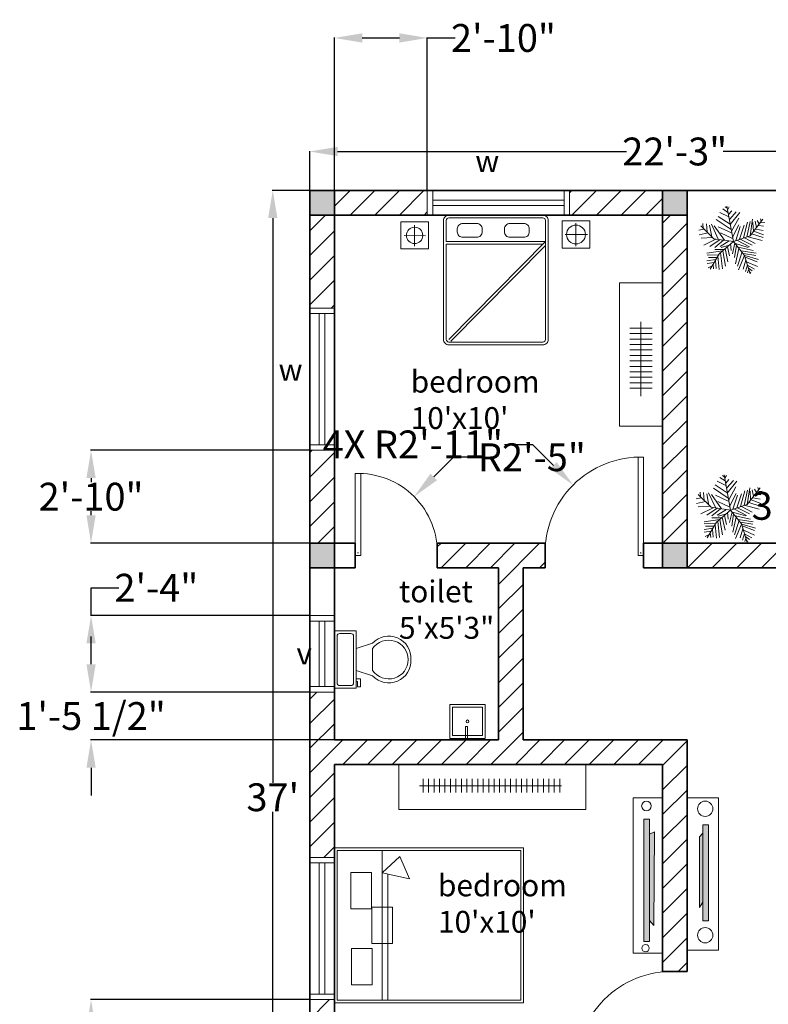
# Model space of a CAD drawing. Units: inches. Extents: x 1222 to 2611, y 176 to 793.
# Tile 2 of 5: x 1223 to 1497, y 433 to 793. Entities that reach past the tile are written whole.
import ezdxf

# ---------------------------------------------------------------- set-up
doc = ezdxf.new("R2010")
doc.units = ezdxf.units.IN
doc.header["$MEASUREMENT"] = 0
for name, color, linetype, lineweight in [('A-ANNO-DIMS', 2, 'Continuous', 18), ('A-ANNO-TEXT', 7, 'Continuous', 25), ('A-AREA-IDEN', 7, 'Continuous', 25), ('A-COLS', 7, 'Continuous', 35), ('A-COLS-PATT', 18, 'Continuous', 13), ('A-DOOR', 3, 'Continuous', 18), ('A-EQPM', 8, 'Continuous', 18), ('A-EQPM-PATT', 18, 'Continuous', 13), ('A-FLOR-CASE', 9, 'Continuous', 18), ('A-FLOR-FIXT', 9, 'Continuous', 18), ('A-FURN', 8, 'Continuous', 18), ('A-GLAZ', 4, 'Continuous', 18), ('A-WALL', 7, 'Continuous', 35), ('A-WALL-PATT', 30, 'Continuous', 13), ('L-PLNT', 94, 'Continuous', 13)]:
    doc.layers.add(name, color=color, linetype=linetype, lineweight=lineweight)
doc.styles.get("Standard").update_dxf_attribs({"font": 'arial.ttf'})
doc.dimstyles.get("Standard").update_dxf_attribs({"dimtxt": 10.18, "dimasz": 10.18, "dimexe": 0.18, "dimexo": 0.0625, "dimgap": 0.09, "dimtad": 0, "dimtih": 1, "dimtoh": 1, "dimdec": 0, "dimzin": 0, "dimdsep": 46, "dimlunit": 3, "dimtxsty": 'Standard', "dimcen": 0.09, "dimadec": 0, "dimazin": 0, "dimtfac": 1, "dimtdec": 0, "dimtofl": 0, "dimtmove": 0, "dimatfit": 3, "dimfxl": 1, "dimtolj": 1, "dimtzin": 0, "dimarcsym": 0})

# ---------------------------------------------------------------- blocks, each defined once
blk = doc.blocks.new('*U2')
for p, q in [((9.5, -6), (9.5, -2)), ((-10, -8.5), (-8, -8.5)), ((-10, -9.5), (-10, -8.5)), ((-7, -9.5), (-10, -9.5)), ((-8, -8.5), (-8, -8)), ((-7, -8), (-7, -9.5)), ((-4, -8), (-6, -14)), ((4, -8), (6, -14)), ((4, -14), (-4, -14))]:
    blk.add_line(p, q)
blk.add_lwpolyline([(10.5, -8), (10.5, 0), (-10.5, 0), (-10.5, -8)], close=True)
for points in [[(-9.5, -2), (-9.5, -6)], [(8.5, -1), (-8.5, -1)], [(-8.5, -7), (8.5, -7)]]:
    blk.add_lwpolyline(points)
for centre, radius, start, end in [((-8.625, -1.875), 0.8839, 81.8699, 188.1301), ((8.625, -1.875), 0.8839, 351.8699, 98.1301), ((-8.625, -6.125), 0.8839, 171.869898, 278.1301), ((8.625, -6.125), 0.8839, 261.8699, 8.1301), ((-0.4772, -19.9188), 8.0953, 133.01722, 273.38), ((0.0374, -19.8731), 7.127, 124.50543, 269.7), ((-0.0373, -19.8731), 7.127, 270.3, 55.4946), ((0.4773, -19.9188), 8.0953, 266.62, 46.9828)]:
    blk.add_arc(centre, radius, start, end)
blk = doc.blocks.new('*U4')
for p, q in [((-8.737, 47.138), (-17.069, 52.711)), ((-10.186, 53.64), (-13.084, 55.962)), ((0, 0), (-10.5, 57)), ((-9.099, 51.782), (-6.563, 55.962)), ((-7.65, 43.423), (-2.578, 49.46)), ((-5.839, 35.992), (4.667, 48.067)), ((-3.665, 19.273), (-27.574, 35.527)), ((-5.114, 28.097), (-24.676, 40.636)), ((-7.288, 39.707), (-21.778, 46.673)), ((-5.114, 27.632), (10.463, 46.673)), ((-2.941, 16.486), (8.652, 37.85)), ((22.055, 7.198), (27.489, 32.277)), ((27, 9), (48, 36)), ((27.127, 9.056), (31.112, 35.992)), ((35.096, 32.741), (37.27, 22.524)), ((38.719, 34.134), (41.979, 28.561)), ((44.153, 36.456), (45.239, 32.741)), ((-47.498, 19.737), (-55.83, 18.344)), ((-31.5, 4.5), (-52.5, 25.5)), ((-48.585, 21.131), (-49.309, 29.026)), ((-43.513, 28.561), (-42.427, 15.558)), ((-38.442, 26.239), (-34.819, 7.663)), ((-35.544, 28.097), (-24.314, 3.947)), ((-14.533, 2.09), (-30.834, 25.31)), ((-24.314, 23.917), (-2.941, 13.7)), ((-1.129, 6.734), (9.014, 26.704)), ((3.942, 1.625), (11.187, 24.381)), ((10.101, 3.483), (17.708, 26.239)), ((16.259, 5.805), (23.142, 31.348)), ((31.836, 30.883), (32.561, 16.486)), ((33.285, 16.486), (48.862, 10.913)), ((36.183, 19.737), (48.137, 17.88)), ((40.53, 25.775), (48.862, 24.846)), ((43.791, 29.954), (51.036, 30.883)), ((-40.615, 13.7), (-55.105, 10.913)), ((-33.37, 6.269), (-52.207, 5.34)), ((-28.299, 3.483), (-47.86, -5.805)), ((-21.416, 3.018), (-38.079, -8.128)), ((0, 0), (-31.5, 4.5)), ((-15.982, 2.09), (-30.11, -9.521)), ((0, 0), (-22.5, -19.5)), ((-6.563, 1.161), (-21.416, -8.128)), ((-20.691, 13.7), (-1.129, 4.876)), ((0, 0), (27, 9)), ((0, 0), (18, -22.5)), ((6.478, 1.625), (26.04, -8.592)), ((11.187, 3.483), (30.749, -5.805)), ((18.07, 5.805), (35.096, -3.483)), ((24.229, 7.663), (46.688, 1.625)), ((29.662, 12.307), (48.137, 6.269)), ((-17.431, -15.094), (-42.789, -18.809)), ((-15.257, -12.772), (-30.11, -12.772)), ((-6.563, -5.805), (-19.967, -9.985)), ((-17.069, -15.094), (-12.721, -40.172)), ((-13.446, -11.378), (-8.737, -32.741)), ((-9.461, -8.592), (-6.201, -23.453)), ((-4.752, -3.483), (-3.665, -14.629)), ((2.493, -3.019), (-1.491, -20.202)), ((1.769, -2.555), (24.229, -9.521)), ((5.029, -6.27), (2.131, -25.775)), ((9.014, -11.378), (3.58, -35.992)), ((7.565, -9.056), (32.198, -14.629)), ((12.274, -15.094), (36.907, -18.809)), ((-28.299, -29.026), (-42.789, -31.348)), ((-24.314, -21.596), (-42.427, -22.06)), ((-26.849, -26.24), (-40.253, -25.775)), ((-22.5, -19.5), (-37.5, -45)), ((-29.023, -30.884), (-27.936, -43.887)), ((-25.038, -23.918), (-22.865, -45.281)), ((-20.691, -18.345), (-17.793, -44.352)), ((14.085, -16.951), (6.478, -40.172)), ((18.07, -22.524), (8.289, -45.745)), ((20.244, -30.419), (15.897, -44.816)), ((16.259, -19.738), (36.183, -22.989)), ((18, -22.5), (27, -52.5)), ((18.433, -22.524), (40.53, -29.026)), ((19.157, -25.311), (38.719, -33.206)), ((-30.834, -34.135), (-42.427, -35.528)), ((-34.457, -39.708), (-40.978, -42.494)), ((-32.646, -36.921), (-31.921, -44.352)), ((22.78, -37.85), (19.519, -48.532)), ((21.331, -32.741), (39.081, -40.636)), ((22.78, -38.314), (34.372, -44.816)), ((24.591, -45.745), (23.142, -50.854)), ((24.591, -43.423), (30.749, -47.603)), ((26.764, -49.925), (28.213, -50.854))]:
    blk.add_line(p, q)
blk = doc.blocks.new('*D9')
at = {"layer": 'A-ANNO-DIMS', "color": 0, "lineweight": -2, "transparency": 16777216}
for p, q in [((1328.8, 730.54), (1328.8, 744.93)), ((1338.98, 744.75), (1444.64, 744.75)), ((1585.62, 744.75), (1479.97, 744.75)), ((1595.8, 730.54), (1595.8, 744.93))]:
    blk.add_line(p, q, dxfattribs=at)
at = {"layer": 'A-ANNO-DIMS', "color": 0, "transparency": 16777216}
for points in [[(1338.98, 746.45), (1338.98, 743.05), (1328.8, 744.75)], [(1585.62, 746.45), (1585.62, 743.05), (1595.8, 744.75)]]:
    blk.add_solid(points, dxfattribs=at)
at = {"layer": 'Defpoints', "color": 0, "transparency": 16777216}
for p in [(1595.8, 744.75), (1328.8, 730.47), (1595.8, 730.47)]:
    blk.add_point(p, dxfattribs=at)
at = {"layer": 'A-ANNO-DIMS', "color": 0, "transparency": 16777216, "insert": (1462.3, 744.75), "char_height": 10.18, "attachment_point": 5}
blk.add_mtext('\\A1;22\'-3"', dxfattribs=at)
blk = doc.blocks.new('*D10')
at = {"layer": 'A-ANNO-DIMS', "color": 0, "lineweight": -2, "transparency": 16777216}
for p, q in [((1328.74, 730.54), (1315.1, 730.54)), ((1315.28, 720.36), (1315.28, 513.8)), ((1315.28, 296.65), (1315.28, 503.21)), ((1328.74, 286.47), (1315.1, 286.47))]:
    blk.add_line(p, q, dxfattribs=at)
at = {"layer": 'A-ANNO-DIMS', "color": 0, "transparency": 16777216}
for points in [[(1313.58, 720.36), (1316.97, 720.36), (1315.28, 730.54)], [(1313.58, 296.65), (1316.97, 296.65), (1315.28, 286.47)]]:
    blk.add_solid(points, dxfattribs=at)
at = {"layer": 'Defpoints', "color": 0, "transparency": 16777216}
for p in [(1315.28, 730.54), (1328.8, 730.54), (1328.8, 286.47)]:
    blk.add_point(p, dxfattribs=at)
at = {"layer": 'A-ANNO-DIMS', "color": 0, "transparency": 16777216, "insert": (1315.28, 508.5), "char_height": 10.18, "attachment_point": 5}
blk.add_mtext("\\A1;37'", dxfattribs=at)
blk = doc.blocks.new('DOOR-SWING-36IN')
for p, q in [((34.01, 0), (34.01, 36)), ((36.01, 0), (36.01, 36)), ((34.01, 0), (36.01, 0))]:
    blk.add_line(p, q)
blk.add_arc((35.01, 1), 35.01, 88.3634, 181.6366)
blk = doc.blocks.new('WINDOW-48IN-PLAN')
for p, q in [((0, 0), (0, 9)), ((2, 0), (2, 9)), ((50, 0), (50, 9)), ((52, 0), (52, 9)), ((2, 5.5), (50, 5.5)), ((2, 3.5), (50, 3.5))]:
    blk.add_line(p, q)
blk = doc.blocks.new('COLUMN-9X9IN')
blk.add_lwpolyline([(0, 9), (9, 9), (9, 0), (0, 0)], close=True)
blk = doc.blocks.new('*D21')
at = {"layer": 'A-ANNO-DIMS', "color": 0, "lineweight": -2, "transparency": 16777216}
for p, q in [((1538.86, 633.25), (1533.3, 633.25)), ((1533.48, 623.07), (1533.48, 620.47)), ((1533.48, 607.15), (1533.48, 609.75)), ((1538.86, 596.97), (1533.3, 596.97))]:
    blk.add_line(p, q, dxfattribs=at)
at = {"layer": 'A-ANNO-DIMS', "color": 0, "transparency": 16777216}
for points in [[(1531.79, 623.07), (1535.18, 623.07), (1533.48, 633.25)], [(1531.79, 607.15), (1535.18, 607.15), (1533.48, 596.97)]]:
    blk.add_solid(points, dxfattribs=at)
at = {"layer": 'Defpoints', "color": 0, "transparency": 16777216}
for p in [(1533.48, 633.25), (1538.92, 633.25), (1538.92, 596.97)]:
    blk.add_point(p, dxfattribs=at)
at = {"layer": 'A-ANNO-DIMS', "color": 0, "transparency": 16777216, "insert": (1533.48, 615.11), "char_height": 10.18, "attachment_point": 5}
blk.add_mtext('\\A1;3\'-0 1/2" TYP.', dxfattribs=at)
blk = doc.blocks.new('*D30')
at = {"layer": 'A-ANNO-DIMS', "color": 0, "lineweight": -2, "transparency": 16777216}
for p, q in [((1337.8, 721.54), (1337.8, 786.47)), ((1347.98, 786.29), (1361.62, 786.29)), ((1371.8, 730.54), (1371.8, 786.47)), ((1371.8, 786.29), (1381.98, 786.29))]:
    blk.add_line(p, q, dxfattribs=at)
at = {"layer": 'A-ANNO-DIMS', "color": 0, "transparency": 16777216}
for points in [[(1347.98, 787.99), (1347.98, 784.59), (1337.8, 786.29)], [(1361.62, 787.99), (1361.62, 784.59), (1371.8, 786.29)]]:
    blk.add_solid(points, dxfattribs=at)
at = {"layer": 'Defpoints', "color": 0, "transparency": 16777216}
for p in [(1371.8, 786.29), (1371.8, 730.47), (1337.8, 721.47)]:
    blk.add_point(p, dxfattribs=at)
at = {"layer": 'A-ANNO-DIMS', "color": 0, "transparency": 16777216, "insert": (1399.65, 786.29), "char_height": 10.18, "attachment_point": 5}
blk.add_mtext('\\A1;2\'-10"', dxfattribs=at)
blk = doc.blocks.new('*D31')
at = {"layer": 'A-ANNO-DIMS', "color": 0, "lineweight": -2, "transparency": 16777216}
for p, q in [((1328.74, 635.47), (1248.62, 635.47)), ((1248.8, 625.29), (1248.8, 623.76)), ((1248.8, 611.65), (1248.8, 613.19)), ((1328.74, 601.47), (1248.62, 601.47))]:
    blk.add_line(p, q, dxfattribs=at)
at = {"layer": 'A-ANNO-DIMS', "color": 0, "transparency": 16777216}
for points in [[(1247.11, 625.29), (1250.5, 625.29), (1248.8, 635.47)], [(1247.11, 611.65), (1250.5, 611.65), (1248.8, 601.47)]]:
    blk.add_solid(points, dxfattribs=at)
at = {"layer": 'Defpoints', "color": 0, "transparency": 16777216}
for p in [(1248.8, 635.47), (1328.8, 635.47), (1328.8, 601.47)]:
    blk.add_point(p, dxfattribs=at)
at = {"layer": 'A-ANNO-DIMS', "color": 0, "transparency": 16777216, "insert": (1248.8, 618.47), "char_height": 10.18, "attachment_point": 5}
blk.add_mtext('\\A1;2\'-10"', dxfattribs=at)
blk = doc.blocks.new('*D32')
at = {"layer": 'A-ANNO-DIMS', "color": 0, "lineweight": -2, "transparency": 16777216}
for p, q in [((1248.8, 557.15), (1248.8, 567.33)), ((1328.74, 546.97), (1248.62, 546.97)), ((1337.74, 529.47), (1248.62, 529.47)), ((1248.8, 519.29), (1248.8, 509.11))]:
    blk.add_line(p, q, dxfattribs=at)
at = {"layer": 'A-ANNO-DIMS', "color": 0, "transparency": 16777216}
for points in [[(1247.11, 557.15), (1250.5, 557.15), (1248.8, 546.97)], [(1247.11, 519.29), (1250.5, 519.29), (1248.8, 529.47)]]:
    blk.add_solid(points, dxfattribs=at)
at = {"layer": 'Defpoints', "color": 0, "transparency": 16777216}
for p in [(1248.8, 546.97), (1328.8, 546.97), (1337.8, 529.47)]:
    blk.add_point(p, dxfattribs=at)
at = {"layer": 'A-ANNO-DIMS', "color": 0, "transparency": 16777216, "insert": (1248.8, 538.22), "char_height": 10.18, "attachment_point": 5}
blk.add_mtext('\\A1;1\'-5 1/2"', dxfattribs=at)
blk = doc.blocks.new('*D33')
at = {"layer": 'A-ANNO-DIMS', "color": 0, "lineweight": -2, "transparency": 16777216}
for p, q in [((1248.8, 574.97), (1248.8, 585.15)), ((1248.8, 585.15), (1258.98, 585.15)), ((1328.74, 574.97), (1248.62, 574.97)), ((1248.8, 557.15), (1248.8, 564.79)), ((1328.74, 546.97), (1248.62, 546.97))]:
    blk.add_line(p, q, dxfattribs=at)
at = {"layer": 'A-ANNO-DIMS', "color": 0, "transparency": 16777216}
for points in [[(1247.11, 564.79), (1250.5, 564.79), (1248.8, 574.97)], [(1247.11, 557.15), (1250.5, 557.15), (1248.8, 546.97)]]:
    blk.add_solid(points, dxfattribs=at)
at = {"layer": 'Defpoints', "color": 0, "transparency": 16777216}
for p in [(1248.8, 574.97), (1328.8, 574.97), (1328.8, 546.97)]:
    blk.add_point(p, dxfattribs=at)
at = {"layer": 'A-ANNO-DIMS', "color": 0, "transparency": 16777216, "insert": (1272.69, 585.15), "char_height": 10.18, "attachment_point": 5}
blk.add_mtext('\\A1;2\'-4"', dxfattribs=at)
blk = doc.blocks.new('*D34')
at = {"layer": 'A-ANNO-DIMS', "color": 0, "lineweight": -2, "transparency": 16777216}
for p, q in [((1328.74, 434.47), (1248.62, 434.47)), ((1248.8, 424.29), (1248.8, 422.76)), ((1248.8, 410.65), (1248.8, 412.19)), ((1328.74, 400.47), (1248.62, 400.47))]:
    blk.add_line(p, q, dxfattribs=at)
at = {"layer": 'A-ANNO-DIMS', "color": 0, "transparency": 16777216}
for points in [[(1247.11, 424.29), (1250.5, 424.29), (1248.8, 434.47)], [(1247.11, 410.65), (1250.5, 410.65), (1248.8, 400.47)]]:
    blk.add_solid(points, dxfattribs=at)
at = {"layer": 'Defpoints', "color": 0, "transparency": 16777216}
for p in [(1248.8, 434.47), (1328.8, 434.47), (1328.8, 400.47)]:
    blk.add_point(p, dxfattribs=at)
at = {"layer": 'A-ANNO-DIMS', "color": 0, "transparency": 16777216, "insert": (1248.8, 417.47), "char_height": 10.18, "attachment_point": 5}
blk.add_mtext('\\A1;2\'-10"', dxfattribs=at)
blk = doc.blocks.new('*D56')
at = {"layer": 'A-ANNO-DIMS', "color": 0, "lineweight": -2, "transparency": 16777216}
for p, q in [((1400.08, 637.59), (1410.26, 637.59)), ((1410.26, 637.59), (1417.91, 629.93)), ((1449.78, 597.97), (1449.96, 597.97)), ((1449.87, 597.88), (1449.87, 598.06))]:
    blk.add_line(p, q, dxfattribs=at)
at = {"layer": 'A-ANNO-DIMS', "color": 0, "transparency": 16777216}
blk.add_solid([(1419.11, 631.13), (1416.71, 628.73), (1425.11, 622.73)], dxfattribs=at)
at = {"layer": 'Defpoints', "color": 0, "transparency": 16777216}
for p in [(1425.11, 622.73), (1449.87, 597.97)]:
    blk.add_point(p, dxfattribs=at)
at = {"layer": 'A-ANNO-DIMS', "color": 0, "transparency": 16777216, "insert": (1366.49, 637.59), "char_height": 10.18, "attachment_point": 5}
blk.add_mtext('\\A1;4X R2\'-11"', dxfattribs=at)
blk = doc.blocks.new('*D57')
at = {"layer": 'A-ANNO-DIMS', "color": 0, "lineweight": -2, "transparency": 16777216}
for p, q in [((1381.37, 632.89), (1374.17, 625.69)), ((1391.55, 632.89), (1381.37, 632.89)), ((1346.36, 597.97), (1346.54, 597.97)), ((1346.45, 597.88), (1346.45, 598.06))]:
    blk.add_line(p, q, dxfattribs=at)
at = {"layer": 'A-ANNO-DIMS', "color": 0, "transparency": 16777216}
blk.add_solid([(1372.97, 626.89), (1375.37, 624.49), (1366.97, 618.49)], dxfattribs=at)
at = {"layer": 'Defpoints', "color": 0, "transparency": 16777216}
for p in [(1366.97, 618.49), (1346.45, 597.97)]:
    blk.add_point(p, dxfattribs=at)
at = {"layer": 'A-ANNO-DIMS', "color": 0, "transparency": 16777216, "insert": (1410.04, 632.89), "char_height": 10.18, "attachment_point": 5}
blk.add_mtext('\\A1;R2\'-5"', dxfattribs=at)

msp = doc.modelspace()

# ---------------------------------------------------------------- hatches: boundary and pattern name
at = {"layer": 'A-COLS-PATT'}
h = msp.add_hatch(color=256, dxfattribs=at)
h.dxf.hatch_style = 1
h.paths.add_polyline_path([(1337.8, 730.47), (1328.8, 730.47), (1328.8, 721.47), (1337.8, 721.47)])
h.paths.add_polyline_path([(1466.8, 730.47), (1457.8, 730.47), (1457.8, 721.47), (1466.8, 721.47)])
h.paths.add_polyline_path([(1595.8, 730.47), (1586.8, 730.47), (1586.8, 721.47), (1595.8, 721.47)])
h.paths.add_polyline_path([(1595.8, 601.42), (1586.8, 601.42), (1586.8, 592.42), (1595.8, 592.42)])
h.paths.add_polyline_path([(1466.8, 601.47), (1457.8, 601.47), (1457.8, 592.47), (1466.8, 592.47)])
h.paths.add_polyline_path([(1337.8, 601.47), (1328.8, 601.47), (1328.8, 592.47), (1337.8, 592.47)])
h.paths.add_polyline_path([(1337.8, 400.47), (1328.8, 400.47), (1328.8, 391.47), (1337.8, 391.47)])
h.paths.add_polyline_path([(1466.8, 400.47), (1457.8, 400.47), (1457.8, 391.47), (1466.8, 391.47)])
h.paths.add_polyline_path([(1595.8, 400.41), (1586.8, 400.41), (1586.8, 391.41), (1595.8, 391.41)])
h.paths.add_polyline_path([(1466.56, 295.47), (1457.56, 295.47), (1457.56, 286.47), (1466.56, 286.47)])
h.paths.add_polyline_path([(1595.8, 295.47), (1586.8, 295.47), (1586.8, 286.47), (1595.8, 286.47)])
h.paths.add_polyline_path([(1337.8, 295.47), (1328.8, 295.47), (1328.8, 286.47), (1337.8, 286.47)])
at = {"layer": 'A-EQPM-PATT'}
h = msp.add_hatch(color=256, dxfattribs=at)
h.dxf.hatch_style = 1
h.paths.add_polyline_path([(1453.1, 500.52), (1450.95, 500.52), (1450.95, 455.73), (1453.1, 455.73)])
h.paths.add_polyline_path([(1454.95, 495.86), (1453.1, 494.94), (1453.1, 463.37), (1454.68, 461.57)])
h = msp.add_hatch(color=256, dxfattribs=at)
h.dxf.hatch_style = 1
h.paths.add_polyline_path([(1474.66, 498.47), (1472.58, 498.47), (1472.58, 463.24), (1474.66, 463.24)])
h.paths.add_polyline_path([(1472.58, 495.4), (1471.4, 494.01), (1471.4, 468.17), (1472.58, 470.11)])
at = {"layer": 'A-WALL-PATT'}
h = msp.add_hatch(dxfattribs=at)
h.set_pattern_fill('ANSI31', color=256, scale=51)
h.paths.add_polyline_path([(1337.8, 721.47), (1328.8, 721.47), (1328.8, 687.47), (1337.8, 687.47)])
h.paths.add_polyline_path([(1337.8, 635.47), (1328.8, 635.47), (1328.8, 601.47), (1337.8, 601.47)])
h.paths.add_polyline_path([(1371.8, 730.47), (1337.8, 730.47), (1337.8, 721.47), (1371.8, 721.47)])
h.paths.add_polyline_path([(1457.8, 730.47), (1423.8, 730.47), (1423.8, 721.47), (1457.8, 721.47)])
h.paths.add_polyline_path([(1466.8, 721.47), (1457.8, 721.47), (1457.8, 601.47), (1466.8, 601.47)])
h.paths.add_polyline_path([(1539.2, 596.97, -0.014283), (1539.2, 598.97), (1539.2, 601.47), (1466.8, 601.47), (1466.8, 592.47), (1539.2, 592.47)])
h.paths.add_polyline_path([(1595.8, 592.42), (1586.8, 592.42), (1586.8, 534.47), (1595.8, 534.47)])
h.paths.add_polyline_path([(1595.8, 458.47), (1586.8, 458.47), (1586.8, 400.41), (1595.8, 400.41)])
h.paths.add_polyline_path([(1595.8, 391.41), (1586.8, 391.41), (1586.8, 369.47), (1595.8, 369.47)])
h.paths.add_polyline_path([(1595.8, 317.47), (1586.8, 317.47), (1586.8, 295.47), (1595.8, 295.47)])
h.paths.add_polyline_path([(1586.8, 295.47), (1552.8, 295.47), (1552.8, 286.47), (1586.8, 286.47)])
h.paths.add_polyline_path([(1500.8, 295.47), (1466.8, 295.47), (1466.8, 349.72), (1462.3, 349.72, -0.014283), (1460.3, 349.72), (1457.8, 349.72), (1457.8, 295.47), (1466.56, 295.47), (1466.56, 286.47), (1500.8, 286.47)])
h.paths.add_polyline_path([(1457.56, 295.47), (1337.8, 295.47), (1337.8, 286.47), (1457.56, 286.47)])
h.paths.add_polyline_path([(1337.8, 317.47), (1328.8, 317.47), (1328.8, 295.47), (1337.8, 295.47)])
h.paths.add_polyline_path([(1337.8, 391.47), (1328.8, 391.47), (1328.8, 369.47), (1337.8, 369.47)])
h.paths.add_polyline_path([(1337.8, 434.47), (1328.8, 434.47), (1328.8, 400.47), (1337.8, 400.47)])
h.paths.add_polyline_path([(1457.8, 400.47), (1337.8, 400.47), (1337.8, 391.47), (1457.8, 391.47)])
h.paths.add_polyline_path([(1546.8, 395.97, -0.014283), (1546.8, 397.97), (1546.8, 400.47), (1466.8, 400.47), (1466.8, 391.47), (1546.8, 391.47)])
h.paths.add_polyline_path([(1466.8, 408.77), (1457.8, 408.77), (1457.8, 400.47), (1466.8, 400.47)])
h.paths.add_polyline_path([(1466.8, 391.47), (1457.8, 391.47), (1457.8, 385.72), (1466.8, 385.72)])
h.paths.add_polyline_path([(1586.8, 400.47), (1582.8, 400.47), (1582.8, 395.97), (1582.8, 391.47), (1586.8, 391.47)])
h.paths.add_polyline_path([(1466.8, 529.47), (1457.8, 529.47), (1406.8, 529.47), (1406.8, 592.47), (1414.87, 592.47), (1414.87, 596.97, -0.014283), (1414.87, 598.97), (1414.87, 601.47), (1375.45, 601.47), (1375.45, 598.97, -0.017236), (1375.45, 596.97), (1375.45, 592.47), (1397.8, 592.47), (1397.8, 529.47), (1337.8, 529.47), (1337.8, 546.97), (1328.8, 546.97), (1328.8, 486.47), (1337.8, 486.47), (1337.8, 490.02), (1337.8, 520.47), (1457.8, 520.47), (1457.8, 444.77), (1460.3, 444.77, -0.014283), (1462.3, 444.77), (1466.8, 444.77)])
h.paths.add_polyline_path([(1457.8, 601.47), (1450.87, 601.47), (1450.87, 596.97), (1450.87, 592.47), (1457.8, 592.47)], flags=0)
h.paths.add_polyline_path([(1586.8, 601.47), (1575.2, 601.47), (1575.2, 596.97), (1575.2, 592.47), (1586.8, 592.47)])

# ---------------------------------------------------------------- linework, layer by layer
at = {"layer": 'A-DOOR'}
for p, q in [((1345.45, 596.97), (1345.45, 626.97)), ((1347.45, 596.97), (1347.45, 626.97)), ((1347.45, 596.97), (1345.45, 596.97))]:
    msp.add_line(p, q, dxfattribs=at)
msp.add_arc((1346.45, 597.97), 29.02, 358.0251, 91.9749, dxfattribs=at)
at = {"layer": 'A-EQPM'}
for p, q in [((1453.1, 494.94), (1454.95, 495.86)), ((1454.95, 495.86), (1454.68, 461.57)), ((1472.58, 495.4), (1471.4, 494.01)), ((1471.4, 494.01), (1471.4, 468.17)), ((1471.4, 468.17), (1472.58, 470.11)), ((1454.68, 461.57), (1453.1, 463.37))]:
    msp.add_line(p, q, dxfattribs=at)
for points in [[(1457.8, 508.28), (1457.8, 508.28), (1447.11, 508.28), (1447.11, 508.28), (1447.11, 451.46), (1447.11, 451.46), (1457.8, 451.46), (1457.8, 451.46)], [(1466.8, 508.28), (1466.8, 508.28), (1478.29, 508.28), (1478.29, 508.28), (1478.29, 452.6), (1478.29, 452.6), (1466.8, 452.6), (1466.8, 452.6)], [(1453.1, 500.52), (1453.1, 500.52), (1450.95, 500.52), (1450.95, 500.52), (1450.95, 455.73), (1450.95, 455.73), (1453.1, 455.73), (1453.1, 455.73)], [(1474.66, 498.47), (1474.66, 498.47), (1472.58, 498.47), (1472.58, 498.47), (1472.58, 463.24), (1472.58, 463.24), (1474.66, 463.24), (1474.66, 463.24)]]:
    msp.add_lwpolyline(points, close=True, dxfattribs=at)
for centre, radius in [((1451.95, 505.32), 1.75), ((1473.43, 504.3), 2.8), ((1473.43, 458.02), 2.8), ((1451.63, 453.31), 1.34)]:
    msp.add_circle(centre, radius, dxfattribs=at)
at = {"layer": 'A-FLOR-CASE'}
for p, q in [((1449.91, 682.43), (1449.91, 655.25)), ((1445.91, 680.13), (1454.06, 680.13)), ((1445.91, 678.13), (1454.06, 678.13)), ((1445.91, 676.13), (1454.06, 676.13)), ((1445.91, 674.13), (1454.06, 674.13)), ((1445.91, 672.13), (1454.06, 672.13)), ((1445.91, 670.13), (1454.06, 670.13)), ((1445.91, 668.13), (1454.06, 668.13)), ((1445.91, 666.13), (1454.06, 666.13)), ((1445.91, 664.13), (1454.06, 664.13)), ((1445.91, 662.13), (1454.06, 662.13)), ((1445.91, 660.13), (1454.06, 660.13)), ((1445.91, 658.13), (1454.06, 658.13)), ((1370.25, 515.22), (1370.25, 510.23)), ((1372.25, 515.22), (1372.25, 510.23)), ((1374.25, 515.22), (1374.25, 510.23)), ((1376.25, 515.22), (1376.25, 510.23)), ((1378.25, 515.22), (1378.25, 510.23)), ((1380.25, 515.22), (1380.25, 510.23)), ((1382.25, 515.22), (1382.25, 510.23)), ((1384.25, 515.22), (1384.25, 510.23)), ((1386.25, 515.22), (1386.25, 510.23)), ((1388.25, 515.22), (1388.25, 510.23)), ((1390.25, 515.22), (1390.25, 510.23)), ((1392.25, 515.22), (1392.25, 510.23)), ((1394.25, 515.22), (1394.25, 510.23)), ((1396.25, 515.22), (1396.25, 510.23)), ((1398.25, 515.22), (1398.25, 510.23)), ((1400.25, 515.22), (1400.25, 510.23)), ((1402.25, 515.22), (1402.25, 510.23)), ((1404.25, 515.22), (1404.25, 510.23)), ((1406.25, 515.22), (1406.25, 510.23)), ((1408.25, 515.22), (1408.25, 510.23)), ((1410.25, 515.22), (1410.25, 510.23)), ((1412.25, 515.22), (1412.25, 510.23)), ((1414.25, 515.22), (1414.25, 510.23)), ((1416.25, 515.22), (1416.25, 510.23)), ((1418.25, 515.22), (1418.25, 510.23)), ((1420.25, 515.22), (1420.25, 510.23)), ((1368.88, 512.68), (1420.85, 512.68))]:
    msp.add_line(p, q, dxfattribs=at)
for points in [[(1457.8, 696.67), (1457.8, 696.67), (1442.08, 696.67), (1442.08, 696.67), (1442.08, 644.23), (1442.08, 644.23), (1457.8, 644.23), (1457.8, 644.23)], [(1442.08, 666.74), (1442.08, 666.74), (1442.08, 666.74), (1442.08, 666.74), (1442.08, 660.81), (1442.08, 660.81), (1442.08, 660.81), (1442.08, 660.81)], [(1361.42, 520.47), (1361.42, 520.47), (1429.78, 520.47), (1429.78, 520.47), (1429.78, 504.01), (1429.78, 504.01), (1361.42, 504.01), (1361.42, 504.01)]]:
    msp.add_lwpolyline(points, close=True, dxfattribs=at)
at = {"layer": 'A-FLOR-FIXT'}
for points in [[(1379.99, 530.06), (1379.99, 530.06), (1392.97, 530.06), (1392.97, 530.06), (1392.97, 542.46), (1392.97, 542.46), (1379.99, 542.46), (1379.99, 542.46)], [(1380.99, 531.06), (1391.97, 531.06), (1391.97, 541.46), (1380.99, 541.46)], [(1386.48, 530.06), (1386.48, 530.06), (1385.8, 530.06), (1385.8, 530.06), (1385.8, 534.33), (1385.8, 534.33), (1386.48, 534.33), (1386.48, 534.33)]]:
    msp.add_lwpolyline(points, close=True, dxfattribs=at)
msp.add_circle((1386.48, 536.26), 0.517, dxfattribs=at)
at = {"layer": 'A-FURN'}
for p, q in [((1367.15, 717.85), (1367.15, 710.08)), ((1426.17, 718.52), (1426.17, 710.13)), ((1363.29, 713.96), (1371.08, 713.88)), ((1422.2, 714.33), (1430.35, 714.33)), ((1378.72, 711.8), (1415.04, 711.8)), ((1378.72, 710.8), (1414.05, 710.8)), ((1415.04, 711.8), (1379.72, 676.03)), ((1415.04, 710.38), (1380.43, 675.33)), ((1355.24, 489.02), (1355.24, 434.26)), ((1355.24, 480.86), (1361.7, 486.84)), ((1361.7, 486.84), (1365.28, 478.6)), ((1365.28, 478.6), (1355.24, 480.86)), ((1357.33, 434.26), (1357.34, 480.39))]:
    msp.add_line(p, q, dxfattribs=at)
for points in [[(1377.72, 719.47, -0.414214), (1379.72, 721.47), (1414.04, 721.47, -0.414214), (1416.04, 719.47), (1416.04, 676.03, -0.414214), (1414.04, 674.03), (1379.72, 674.03, -0.414214), (1377.72, 676.03)], [(1382.77, 716.41, -0.414214), (1384.77, 718.41), (1389.87, 718.41, -0.414214), (1391.87, 716.41), (1391.87, 715.36, -0.414214), (1389.87, 713.36), (1384.77, 713.36, -0.414214), (1382.77, 715.36)], [(1400.01, 716.41, -0.414214), (1402.01, 718.41), (1407.11, 718.41, -0.414214), (1409.11, 716.41), (1409.11, 715.36, -0.414214), (1407.11, 713.36), (1402.01, 713.36, -0.414214), (1400.01, 715.36)]]:
    msp.add_lwpolyline(points, format="xyb", close=True, dxfattribs=at)
msp.add_lwpolyline([(1378.72, 711.8), (1378.72, 719.47, -0.414214), (1379.72, 720.47), (1414.04, 720.47, -0.414214), (1415.04, 719.47), (1415.04, 676.03, -0.414214), (1414.04, 675.03), (1379.72, 675.03, -0.414214), (1378.72, 676.03), (1378.72, 710.8)], format="xyb", dxfattribs=at)
for points in [[(1362.12, 719), (1362.12, 719), (1372.18, 719), (1372.18, 719), (1372.18, 709.09), (1372.18, 709.09), (1362.12, 709.09), (1362.12, 709.09)], [(1421.14, 719.33), (1421.14, 719.33), (1431.2, 719.33), (1431.2, 719.33), (1431.2, 709.42), (1431.2, 709.42), (1421.14, 709.42), (1421.14, 709.42)], [(1337.8, 490.02), (1337.8, 490.02), (1406.99, 490.02), (1406.99, 490.02), (1406.99, 433.26), (1406.99, 433.26), (1337.8, 433.26), (1337.8, 433.26)], [(1338.8, 489.02), (1405.99, 489.02), (1405.99, 434.26), (1338.8, 434.26)], [(1343.88, 480.97), (1343.88, 480.97), (1351.44, 480.97), (1351.44, 480.97), (1351.44, 467.69), (1351.44, 467.69), (1343.88, 467.69), (1343.88, 467.69)], [(1351.46, 468.28), (1351.46, 468.28), (1359.02, 468.28), (1359.02, 468.28), (1359.02, 455), (1359.02, 455), (1351.46, 455), (1351.46, 455)], [(1344.11, 453.18), (1344.11, 453.18), (1351.67, 453.18), (1351.67, 453.18), (1351.67, 439.9), (1351.67, 439.9), (1344.11, 439.9), (1344.11, 439.9)]]:
    msp.add_lwpolyline(points, close=True, dxfattribs=at)
for centre, radius in [((1367.15, 714.04), 2.99), ((1426.17, 714.37), 3.46)]:
    msp.add_circle(centre, radius, dxfattribs=at)
at = {"layer": 'A-GLAZ'}
for p, q in [((1373.8, 725.97), (1373.8, 725.97)), ((1337.8, 574.97), (1328.8, 574.97)), ((1337.8, 572.97), (1328.8, 572.97)), ((1332.3, 572.97), (1332.3, 548.97)), ((1334.3, 572.97), (1334.3, 548.97)), ((1337.8, 548.97), (1328.8, 548.97)), ((1337.8, 546.97), (1328.8, 546.97))]:
    msp.add_line(p, q, dxfattribs=at)
at = {"layer": 'A-WALL'}
for p, q in [((1328.8, 286.47), (1328.8, 730.47)), ((1328.8, 730.47), (1595.8, 730.47)), ((1337.8, 721.47), (1457.8, 721.47)), ((1337.8, 601.47), (1337.8, 721.47)), ((1457.8, 601.47), (1457.8, 721.47)), ((1457.8, 601.47), (1457.8, 721.47)), ((1466.8, 601.47), (1466.8, 721.47)), ((1466.8, 601.47), (1466.8, 721.47)), ((1337.8, 601.47), (1345.45, 601.47)), ((1345.45, 601.47), (1345.45, 592.47)), ((1375.45, 601.47), (1414.87, 601.47)), ((1375.45, 601.47), (1375.45, 592.47)), ((1414.87, 601.47), (1414.87, 592.47)), ((1450.87, 601.47), (1450.87, 592.47)), ((1450.87, 601.47), (1457.8, 601.47)), ((1466.8, 601.47), (1539.2, 601.47)), ((1337.8, 592.47), (1345.45, 592.47)), ((1337.8, 529.47), (1337.8, 592.47)), ((1375.45, 592.47), (1397.8, 592.47)), ((1397.8, 529.47), (1397.8, 592.47)), ((1406.8, 529.47), (1406.8, 592.47)), ((1406.8, 592.47), (1414.87, 592.47)), ((1450.87, 592.47), (1457.8, 592.47)), ((1457.8, 592.47), (1466.8, 592.47)), ((1466.8, 592.47), (1539.2, 592.47)), ((1337.8, 529.47), (1397.8, 529.47)), ((1406.8, 529.47), (1457.8, 529.47)), ((1457.8, 529.47), (1466.8, 529.47)), ((1466.8, 444.77), (1466.8, 529.47)), ((1337.8, 520.47), (1457.8, 520.47)), ((1337.8, 400.47), (1337.8, 520.47)), ((1457.8, 444.77), (1457.8, 520.47)), ((1457.8, 444.77), (1466.8, 444.77))]:
    msp.add_line(p, q, dxfattribs=at)

# ---------------------------------------------------------------- block references
at = {"layer": 'A-COLS'}
for p in [(1328.8, 721.47), (1457.8, 721.47), (1328.8, 592.47), (1457.8, 592.47)]:
    msp.add_blockref('COLUMN-9X9IN', p, dxfattribs=at)
at = {"layer": 'A-DOOR'}
msp.add_blockref('DOOR-SWING-36IN', (1414.86, 596.97), dxfattribs=at)
at = {"layer": 'A-DOOR', "extrusion": (0, 0, -1), "zscale": -1, "rotation": 270.0000000000005}
msp.add_blockref('DOOR-SWING-36IN', (-1462.3, 444.78), dxfattribs=at)
at = {"layer": 'A-FLOR-FIXT', "rotation": 90}
msp.add_blockref('*U2', (1337.8, 558.88), dxfattribs=at)
at = {"layer": 'A-GLAZ'}
msp.add_blockref('WINDOW-48IN-PLAN', (1371.8, 721.47), dxfattribs=at)
for p, rotation in [((1337.8, 635.47), 89.99999999999879), ((1337.8, 434.47), 89.99999999999883)]:
    msp.add_blockref('WINDOW-48IN-PLAN', p, dxfattribs=dict(at, rotation=rotation))
at = {"layer": 'L-PLNT', "xscale": 0.225926009387716, "yscale": 0.225926009387716, "zscale": 0.225926009387716}
for p in [(1483.73, 711.84), (1482.69, 613.56)]:
    msp.add_blockref('*U4', p, dxfattribs=at)

# ---------------------------------------------------------------- texts
at = {"layer": 'A-ANNO-TEXT', "char_height": 8, "attachment_point": 1}
for s, insert in [('w', (1389.34, 745.22)), ('w', (1317.4, 668.85)), ('v', (1323.93, 565.11))]:
    msp.add_mtext_dynamic_manual_height_columns(s, width=4.8776, gutter_width=1, heights=[0], dxfattribs=dict(at, insert=insert))
at = {"layer": 'A-AREA-IDEN', "char_height": 8, "attachment_point": 1}
for s, insert in [("bedroom\\P10'x10'", (1365.73, 664.56)), ('toilet\\P5\'x5\'3"', (1361.44, 587.82)), ("bedroom\\P10'x10'", (1375.7, 480.27))]:
    msp.add_mtext_dynamic_manual_height_columns(s, width=78.0148, gutter_width=1, heights=[0], dxfattribs=dict(at, insert=insert))

# ---------------------------------------------------------------- dimensions: what is measured, and where the dimension line sits
at = {"layer": 'A-ANNO-DIMS'}
for base, p1, p2, override, picture, middle in [((1371.8, 786.29), (1337.8, 721.47), (1371.8, 730.47), {"dimdec": 1, "dimlfac": 1, "dimrnd": 0, "dimzin": 1, "dimdsep": 46, "dimlunit": 4, "dimfrac": 2}, '*D30', (1399.65, 786.29)), ((1595.8, 744.75), (1328.8, 730.47), (1595.8, 730.47), {"dimclrd": 0, "dimclre": 0, "dimclrt": 0}, '*D9', (1462.3, 744.75))]:
    dim = msp.add_linear_dim(base=base, p1=p1, p2=p2, dimstyle='Standard', override=override, dxfattribs=at)
    dim.commit()
    dim.dimension.update_dxf_attribs({"geometry": picture, "text_midpoint": middle})
for base, p1, p2, override, picture, middle in [((1315.28, 730.54), (1328.8, 286.47), (1328.8, 730.54), {"dimclrd": 0, "dimclre": 0, "dimclrt": 0}, '*D10', (1315.28, 508.5)), ((1248.8, 635.47), (1328.8, 601.47), (1328.8, 635.47), {"dimdec": 1, "dimlfac": 1, "dimrnd": 0, "dimzin": 1, "dimdsep": 46, "dimlunit": 4, "dimfrac": 2}, '*D31', (1248.8, 618.47)), ((1248.8, 574.97), (1328.8, 546.97), (1328.8, 574.97), {"dimdec": 1, "dimlfac": 1, "dimrnd": 0, "dimzin": 1, "dimdsep": 46, "dimlunit": 4, "dimfrac": 2}, '*D33', (1272.69, 585.15)), ((1248.8, 546.97), (1337.8, 529.47), (1328.8, 546.97), {"dimdec": 1, "dimlfac": 1, "dimrnd": 0, "dimzin": 1, "dimdsep": 46, "dimlunit": 4, "dimfrac": 2}, '*D32', (1248.8, 538.22)), ((1248.8, 434.47), (1328.8, 400.47), (1328.8, 434.47), {"dimdec": 1, "dimlfac": 1, "dimrnd": 0, "dimzin": 1, "dimdsep": 46, "dimlunit": 4, "dimfrac": 2}, '*D34', (1248.8, 417.47))]:
    dim = msp.add_linear_dim(base=base, p1=p1, p2=p2, angle=90, dimstyle='Standard', override=override, dxfattribs=at)
    dim.commit()
    dim.dimension.update_dxf_attribs({"geometry": picture, "text_midpoint": middle})
dim = msp.add_radius_dim(center=(1449.87, 597.97), mpoint=(1425.11, 622.73), text='4X <>', dimstyle='Standard', override={"dimdec": 1, "dimlfac": 1, "dimrnd": 0, "dimzin": 1, "dimdsep": 46, "dimlunit": 4, "dimfrac": 2}, dxfattribs=at)
dim.commit()
dim.dimension.update_dxf_attribs({"geometry": '*D56', "text_midpoint": (1366.49, 637.59), "dimtype": 164})
dim = msp.add_radius_dim(center=(1346.45, 597.97), mpoint=(1366.97, 618.49), dimstyle='Standard', override={"dimdec": 1, "dimlfac": 1, "dimrnd": 0, "dimzin": 1, "dimdsep": 46, "dimlunit": 4, "dimfrac": 2}, dxfattribs=at)
dim.commit()
dim.dimension.update_dxf_attribs({"geometry": '*D57', "text_midpoint": (1410.04, 632.89)})
dim = msp.add_linear_dim(base=(1533.48, 633.25), p1=(1538.92, 596.97), p2=(1538.92, 633.25), angle=90, text='<> TYP.', dimstyle='Standard', override={"dimdec": 1, "dimlfac": 1, "dimrnd": 0, "dimzin": 1, "dimdsep": 46, "dimlunit": 4, "dimfrac": 2}, dxfattribs=at)
dim.commit()
dim.dimension.update_dxf_attribs({"geometry": '*D21', "text_midpoint": (1533.48, 615.11)})

doc.saveas('drawing.dxf')
